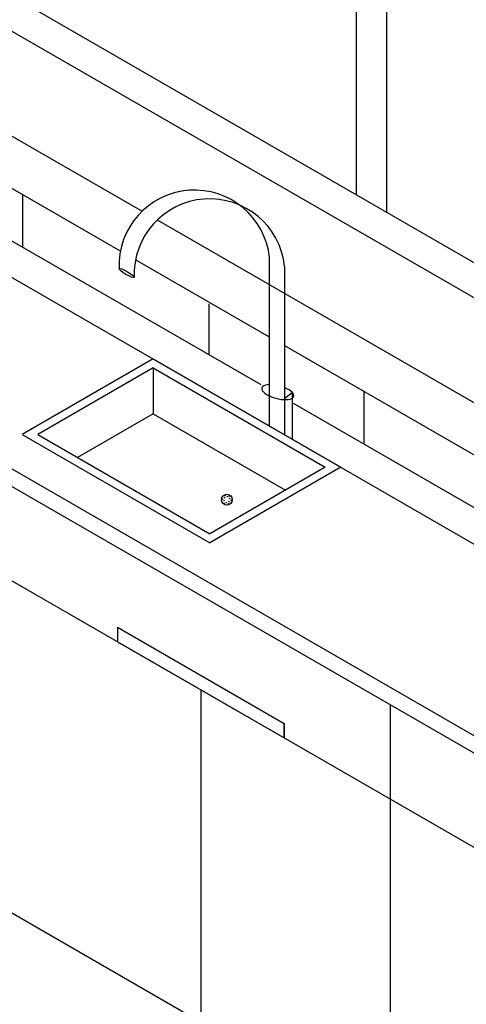
# Model space of a CAD drawing. Units: inches. Extents: x 5770 to 11891, y 3254 to 6808.
# Tile 7 of 15: x 6009 to 6034, y 3403 to 3459. Entities that reach past the tile are written whole.
import ezdxf

# ---------------------------------------------------------------- set-up
doc = ezdxf.new("R2010")
doc.units = ezdxf.units.IN
for name, color, linetype, lineweight in [('A-ANNO-DIMS', 2, 'Continuous', 18), ('A-FURN', 8, 'Continuous', 25), ('A-GLAZ', 4, 'Continuous', 25)]:
    doc.layers.add(name, color=color, linetype=linetype, lineweight=lineweight)
doc.styles.get("Standard").update_dxf_attribs({"font": 'arial.ttf'})
doc.dimstyles.new('ISO-25', dxfattribs={"dimtxt": 2.5, "dimasz": 2.5, "dimexe": 1.25, "dimexo": 0.625, "dimtad": 1, "dimdec": 0, "dimlunit": 3, "dimtxsty": 'Standard', "dimcen": 2.5, "dimadec": 0, "dimazin": 0, "dimtfac": 1, "dimtdec": 0, "dimtmove": 0, "dimatfit": 3, "dimfxl": 1, "dimarcsym": 0})

# ---------------------------------------------------------------- blocks, each defined once
blk = doc.blocks.new('*D7')
at = {"layer": 'A-ANNO-DIMS', "color": 0, "lineweight": -2, "transparency": 16777216}
for p, q in [((5959.627, 3549.37), (5966.461, 3561.208)), ((5968.001, 3558.875), (6136.876, 3461.375)), ((6132.832, 3449.37), (6139.666, 3461.208))]:
    blk.add_line(p, q, dxfattribs=at)
at = {"layer": 'A-ANNO-DIMS', "color": 0, "transparency": 16777216}
for points in [[(5968.21, 3559.236), (5967.793, 3558.514), (5965.836, 3560.125)], [(6137.085, 3461.736), (6136.668, 3461.014), (6139.041, 3460.125)]]:
    blk.add_solid(points, dxfattribs=at)
at = {"layer": 'Defpoints', "color": 0, "transparency": 16777216}
for p in [(5959.314, 3548.829), (6139.041, 3460.125), (6132.519, 3448.829)]:
    blk.add_point(p, dxfattribs=at)
at = {"layer": 'A-ANNO-DIMS', "color": 0, "transparency": 16777216, "insert": (6061.618, 3507.021), "char_height": 2.5, "attachment_point": 5, "rotation": 330}
blk.add_mtext('16\'-8"', dxfattribs=at)
blk = doc.blocks.new('*U8')
blk.add_circle((0, 0), 0.0169)
blk = doc.blocks.new('*U9')
at = {"layer": 'A-FURN', "color": 0, "linetype": 'ByBlock', "lineweight": -2, "transparency": 16777216}
blk.add_blockref('*U8', (3105.418, 1768.292), dxfattribs=at)
for p, rotation in [((3105.673, 1768.264), 299.9999999999999), ((3105.266, 1768.085), 59.99999999999999), ((3105.37, 1767.85), 119.9999999999999), ((3105.625, 1767.823), 180), ((3105.776, 1768.03), 240)]:
    blk.add_blockref('*U8', p, dxfattribs=dict(at, rotation=rotation))
blk = doc.blocks.new('*U10')
blk.add_circle((0, 0), 0.0132)
blk = doc.blocks.new('*U11')
at = {"layer": 'A-FURN', "color": 0, "linetype": 'ByBlock', "lineweight": -2, "transparency": 16777216}
for p, rotation in [((3105.554, 1768.228), 300), ((3105.357, 1768), 59.99999999999997), ((3105.489, 1767.887), 120), ((3105.653, 1767.944), 180), ((3105.686, 1768.114), 240)]:
    blk.add_blockref('*U10', p, dxfattribs=dict(at, rotation=rotation))
blk.add_blockref('*U10', (3105.39, 1768.171), dxfattribs=at)
blk = doc.blocks.new('CABINET-PULL')
for p, q in [((0, 6.322), (9.524, 0.823)), ((0, 6.322), (0, 5.499)), ((0, 6.322), (0, 5.499)), ((0, 5.499), (9.524, 0)), ((9.524, 0.823), (9.524, 0)), ((9.524, 0), (9.524, 0.823))]:
    blk.add_line(p, q)

msp = doc.modelspace()

# ---------------------------------------------------------------- linework, layer by layer
at = {"layer": 'A-FURN'}
for p, q in [((5975.971, 3462.811), (6056.394, 3416.379)), ((5975.971, 3451.863), (6059.32, 3403.741)), ((5975.971, 3450.863), (6059.32, 3402.741)), ((6022.299, 3438.144), (6002.599, 3449.517)), ((6016.362, 3447.572), (6044.169, 3431.517)), ((6022.773, 3440.87), (6015.122, 3445.287)), ((6022.773, 3435.79), (6022.773, 3445.42)), ((6023.639, 3435.29), (6023.639, 3444.92)), ((5979.292, 3443.56), (6059.32, 3397.356)), ((6019.303, 3442.78), (6019.303, 3439.874)), ((6044.169, 3428.517), (6023.639, 3440.37)), ((6016.127, 3439.627), (6008.649, 3435.31)), ((6016.127, 3439.627), (6026.85, 3433.436)), ((6016.127, 3439.111), (6009.543, 3435.31)), ((6016.127, 3439.111), (6016.127, 3436.49)), ((6016.127, 3439.111), (6025.957, 3433.436)), ((6023.639, 3437.394), (6024.073, 3437.71)), ((6024.073, 3437.71), (6024.073, 3435.039)), ((6028.154, 3437.763), (6028.154, 3434.763)), ((6044.169, 3425.517), (6024.15, 3437.075)), ((6016.127, 3436.49), (6011.812, 3433.999)), ((6016.127, 3436.49), (6023.687, 3432.125)), ((6008.649, 3435.31), (6019.372, 3429.118)), ((6009.543, 3435.31), (6019.372, 3429.634)), ((6026.85, 3433.436), (6019.372, 3429.118)), ((6025.957, 3433.436), (6019.372, 3429.634)), ((5964.711, 3432.996), (6059.32, 3378.374)), ((6018.855, 3420.735), (6018.855, 3401.753)), ((6029.662, 3419.864), (6029.662, 3395.496))]:
    msp.add_line(p, q, dxfattribs=at)
msp.add_circle((6020.337, 3431.584), 0.31, dxfattribs=at)
for centre in [(6018.487, 3444.969), (6019.353, 3444.469)]:
    msp.add_arc(centre, 4.309, 6.0073, 182.4039, dxfattribs=at)
msp.add_ellipse((6014.614, 3444.539), major_axis=(0.433, -0.25), ratio=0.175848, dxfattribs=at)
msp.add_ellipse((6023.244, 3437.733), major_axis=(0.909, -0.238), ratio=0.393852, start_param=2.216201, end_param=7.510884, dxfattribs=at)
at = {"layer": 'A-GLAZ'}
for p, q in [((6027.714, 3487.017), (6027.714, 3449.017)), ((6029.446, 3486.017), (6029.446, 3448.017)), ((6009.528, 3459.517), (6047.633, 3437.517)), ((6007.795, 3458.517), (6049.365, 3434.517)), ((6002.599, 3455.517), (6015.496, 3448.072)), ((6014.256, 3445.787), (6002.599, 3452.517)), ((6008.675, 3449.009), (6008.675, 3446.009))]:
    msp.add_line(p, q, dxfattribs=at)

# ---------------------------------------------------------------- block references
at = {"layer": 'A-FURN'}
for name, p in [('*U9', (2914.815, 1663.526)), ('*U11', (2914.815, 1663.526)), ('CABINET-PULL', (6014.093, 3417.969))]:
    msp.add_blockref(name, p, dxfattribs=at)

# ---------------------------------------------------------------- dimensions: what is measured, and where the dimension line sits
at = {"layer": 'A-ANNO-DIMS'}
dim = msp.add_linear_dim(base=(6139.041, 3460.125), p1=(5959.314, 3548.829), p2=(6132.519, 3448.829), angle=330, dimstyle='ISO-25', override={"dimclrd": 0, "dimclre": 0, "dimclrt": 0}, dxfattribs=at)
dim.commit()
dim.dimension.update_dxf_attribs({"geometry": '*D7', "text_midpoint": (6060.667, 3505.374), "dimtype": 161})

doc.saveas('drawing.dxf')
